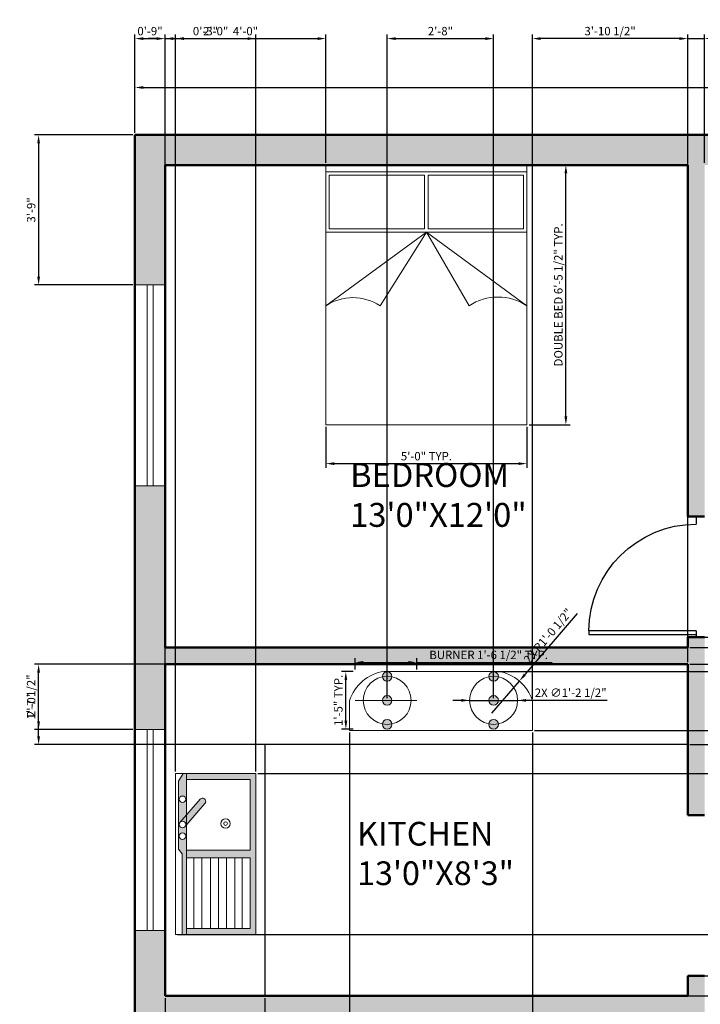
# Model space of a CAD drawing. Units: inches. Extents: x 457 to 882, y 0 to 1111.
# Tile 3 of 4: x 457 to 660, y 817 to 1111. Entities that reach past the tile are written whole.
import ezdxf

# ---------------------------------------------------------------- set-up
doc = ezdxf.new("R2010")
doc.units = ezdxf.units.IN
for name, color, linetype, lineweight in [('A-ANNO-DIMS', 2, 'Continuous', 18), ('A-AREA-IDEN', 7, 'Continuous', 25), ('A-DOOR', 3, 'Continuous', 25), ('A-EQPM', 9, 'Continuous', 18), ('A-FLOR-CASE', 8, 'Continuous', 25), ('A-FLOR-FIXT', 8, 'Continuous', 18), ('A-FLOR-FIXT-PATT', 8, 'Continuous', 13), ('A-FURN', 8, 'Continuous', 18), ('A-GLAZ', 5, 'Continuous', 18), ('A-WALL', 7, 'Continuous', 50), ('A-WALL-PATT', 252, 'Continuous', 13)]:
    doc.layers.add(name, color=color, linetype=linetype, lineweight=lineweight)
doc.styles.get("Standard").update_dxf_attribs({"font": 'arial.ttf'})
doc.dimstyles.new('ISO-25', dxfattribs={"dimtxt": 2.5, "dimasz": 2.5, "dimexe": 1.25, "dimexo": 0.625, "dimtad": 1, "dimdec": 0, "dimlunit": 3, "dimtxsty": 'Standard', "dimcen": 2.5, "dimadec": 0, "dimazin": 0, "dimtfac": 1, "dimtdec": 0, "dimtmove": 0, "dimatfit": 3, "dimfxl": 1, "dimarcsym": 0})

# ---------------------------------------------------------------- blocks, each defined once
blk = doc.blocks.new('*D2')
at = {"layer": 'A-ANNO-DIMS', "color": 0, "lineweight": -2, "transparency": 16777216}
for p, q in [((491.26, 1077.13), (491.26, 1091.91)), ((493.76, 1090.66), (848.76, 1090.66)), ((851.26, 1077.13), (851.26, 1091.91))]:
    blk.add_line(p, q, dxfattribs=at)
at = {"layer": 'A-ANNO-DIMS', "color": 0, "transparency": 16777216}
for points in [[(493.76, 1091.08), (493.76, 1090.24), (491.26, 1090.66)], [(848.76, 1091.08), (848.76, 1090.24), (851.26, 1090.66)]]:
    blk.add_solid(points, dxfattribs=at)
at = {"layer": 'Defpoints', "color": 0, "transparency": 16777216}
for p in [(851.26, 1090.66), (491.26, 1076.51), (851.26, 1076.51)]:
    blk.add_point(p, dxfattribs=at)
at = {"layer": 'A-ANNO-DIMS', "color": 0, "transparency": 16777216, "insert": (671.26, 1092.56), "char_height": 2.5, "attachment_point": 5}
blk.add_mtext("30'", dxfattribs=at)
blk = doc.blocks.new('BED-DOUBLE-60')
for p, q in [((0, 77.49), (0, 0)), ((60, 77.49), (0, 77.49)), ((60, 0), (60, 77.49)), ((60, 75.49), (0, 75.49)), ((29.44, 74.49), (0.94, 74.49)), ((0.94, 74.49), (0.94, 58.49)), ((29.44, 74.49), (29.44, 58.49)), ((59, 74.49), (30.53, 74.49)), ((30.53, 74.49), (30.53, 58.49)), ((59, 74.49), (59, 58.49)), ((60, 57.49), (0, 57.49)), ((30, 57.49), (0, 35.49)), ((29.44, 58.49), (0.94, 58.49)), ((30, 57.49), (16.16, 35.49)), ((60, 35.49), (30, 57.49)), ((30, 57.49), (42.73, 35.49)), ((59, 58.49), (30.53, 58.49)), ((0, 0), (60, 0))]:
    blk.add_line(p, q)
for centre, radius, start, end in [((8.08, 23.34), 14.59, 56.3669, 123.6331), ((51.36, 22.4), 15.69, 56.5972, 123.4028)]:
    blk.add_arc(centre, radius, start, end)
blk = doc.blocks.new('WIN-60-GLAZING')
for p, q in [((0, 0), (0, 60)), ((1.86, 0), (1.86, 60))]:
    blk.add_line(p, q)
blk = doc.blocks.new('DOOR-32-SWING')
for p, q in [((0, 36), (0, 33.7)), ((0, 1.85), (32, 1.85)), ((0, 1.85), (0, 0))]:
    blk.add_line(p, q)
blk.add_arc((0, 1.7), 32, 0.2643, 90)
blk = doc.blocks.new('COOKTOP-BURNER')
for q in [(0, 8.58), (18.39, 8.58)]:
    blk.add_line((9.57, 8.58), q)
for centre, radius in [((9.57, 8.58), 7.15), ((9.57, 15.73), 1.43), ((9.57, 8.58), 1.43), ((9.57, 1.43), 1.43)]:
    blk.add_circle(centre, radius)
blk = doc.blocks.new('*D16')
at = {"layer": 'A-ANNO-DIMS', "color": 0, "lineweight": -2, "transparency": 16777216}
for p, q in [((608.88, 1067.51), (621.13, 1067.51)), ((619.88, 992.51), (619.88, 1065.01)), ((608.88, 990.01), (621.13, 990.01))]:
    blk.add_line(p, q, dxfattribs=at)
at = {"layer": 'A-ANNO-DIMS', "color": 0, "transparency": 16777216}
for points in [[(619.46, 1065.01), (620.3, 1065.01), (619.88, 1067.51)], [(619.46, 992.51), (620.3, 992.51), (619.88, 990.01)]]:
    blk.add_solid(points, dxfattribs=at)
at = {"layer": 'Defpoints', "color": 0, "transparency": 16777216}
for p in [(608.26, 1067.51), (619.88, 1067.51), (608.26, 990.01)]:
    blk.add_point(p, dxfattribs=at)
at = {"layer": 'A-ANNO-DIMS', "color": 0, "transparency": 16777216, "insert": (617.96, 1028.76), "char_height": 2.5, "attachment_point": 5, "rotation": 90}
blk.add_mtext('DOUBLE BED 6\'-5 1/2" TYP.', dxfattribs=at)
blk = doc.blocks.new('*D17')
at = {"layer": 'A-ANNO-DIMS', "color": 0, "lineweight": -2, "transparency": 16777216}
for p, q in [((548.26, 989.39), (548.26, 977.14)), ((608.26, 989.39), (608.26, 977.14)), ((550.76, 978.39), (605.76, 978.39))]:
    blk.add_line(p, q, dxfattribs=at)
at = {"layer": 'A-ANNO-DIMS', "color": 0, "transparency": 16777216}
for points in [[(550.76, 978.8), (550.76, 977.97), (548.26, 978.39)], [(605.76, 978.8), (605.76, 977.97), (608.26, 978.39)]]:
    blk.add_solid(points, dxfattribs=at)
at = {"layer": 'Defpoints', "color": 0, "transparency": 16777216}
for p in [(548.26, 990.01), (608.26, 990.01), (608.26, 978.39)]:
    blk.add_point(p, dxfattribs=at)
at = {"layer": 'A-ANNO-DIMS', "color": 0, "transparency": 16777216, "insert": (578.26, 980.29), "char_height": 2.5, "attachment_point": 5}
blk.add_mtext('5\'-0" TYP.', dxfattribs=at)
blk = doc.blocks.new('*D22')
at = {"layer": 'A-ANNO-DIMS', "color": 0, "lineweight": -2, "transparency": 16777216}
for p, q in [((556.97, 916.92), (556.97, 920.31)), ((575.37, 916.92), (575.37, 920.31)), ((559.47, 919.06), (572.87, 919.06)), ((575.37, 919.06), (615.79, 919.06))]:
    blk.add_line(p, q, dxfattribs=at)
at = {"layer": 'A-ANNO-DIMS', "color": 0, "transparency": 16777216}
for points in [[(559.47, 919.48), (559.47, 918.64), (556.97, 919.06)], [(572.87, 919.48), (572.87, 918.64), (575.37, 919.06)]]:
    blk.add_solid(points, dxfattribs=at)
at = {"layer": 'Defpoints', "color": 0, "transparency": 16777216}
for p in [(575.37, 919.06), (556.97, 916.3), (575.37, 916.3)]:
    blk.add_point(p, dxfattribs=at)
at = {"layer": 'A-ANNO-DIMS', "color": 0, "transparency": 16777216, "insert": (596.83, 920.98), "char_height": 2.5, "attachment_point": 5}
blk.add_mtext('BURNER 1\'-6 1/2" TYP.', dxfattribs=at)
blk = doc.blocks.new('*D23')
at = {"layer": 'A-ANNO-DIMS', "color": 0, "lineweight": -2, "transparency": 16777216}
for p, q in [((556.35, 916.3), (552.96, 916.3)), ((554.21, 901.64), (554.21, 913.8)), ((556.35, 899.14), (552.96, 899.14))]:
    blk.add_line(p, q, dxfattribs=at)
at = {"layer": 'A-ANNO-DIMS', "color": 0, "transparency": 16777216}
for points in [[(553.8, 913.8), (554.63, 913.8), (554.21, 916.3)], [(553.8, 901.64), (554.63, 901.64), (554.21, 899.14)]]:
    blk.add_solid(points, dxfattribs=at)
at = {"layer": 'Defpoints', "color": 0, "transparency": 16777216}
for p in [(554.21, 916.3), (556.97, 916.3), (556.97, 899.14)]:
    blk.add_point(p, dxfattribs=at)
at = {"layer": 'A-ANNO-DIMS', "color": 0, "transparency": 16777216, "insert": (552.31, 907.72), "char_height": 2.5, "attachment_point": 5, "rotation": 90}
blk.add_mtext('1\'-5" TYP.', dxfattribs=at)
blk = doc.blocks.new('*D27')
at = {"layer": 'A-ANNO-DIMS', "color": 0, "lineweight": -2, "transparency": 16777216}
for p, q in [((685.01, 929.13), (685.01, 931.63)), ((656.88, 926.63), (686.26, 926.63)), ((685.01, 926.63), (685.01, 923.51)), ((656.88, 923.51), (686.26, 923.51)), ((685.01, 921.01), (685.01, 910.61))]:
    blk.add_line(p, q, dxfattribs=at)
at = {"layer": 'A-ANNO-DIMS', "color": 0, "transparency": 16777216}
for points in [[(684.59, 929.13), (685.42, 929.13), (685.01, 926.63)], [(684.59, 921.01), (685.42, 921.01), (685.01, 923.51)]]:
    blk.add_solid(points, dxfattribs=at)
at = {"layer": 'Defpoints', "color": 0, "transparency": 16777216}
for p in [(656.26, 926.63), (656.26, 923.51), (685.01, 923.51)]:
    blk.add_point(p, dxfattribs=at)
at = {"layer": 'A-ANNO-DIMS', "color": 0, "transparency": 16777216, "insert": (683.11, 914.56), "char_height": 2.5, "attachment_point": 5, "rotation": 90}
blk.add_mtext('0\'-3"', dxfattribs=at)
blk = doc.blocks.new('*D28')
at = {"layer": 'A-ANNO-DIMS', "color": 0, "lineweight": -2, "transparency": 16777216}
for p, q in [((491.26, 1077.13), (491.26, 1106.51)), ((493.76, 1105.26), (497.76, 1105.26)), ((500.26, 1068.13), (500.26, 1106.51))]:
    blk.add_line(p, q, dxfattribs=at)
at = {"layer": 'A-ANNO-DIMS', "color": 0, "transparency": 16777216}
for points in [[(493.76, 1105.67), (493.76, 1104.84), (491.26, 1105.26)], [(497.76, 1105.67), (497.76, 1104.84), (500.26, 1105.26)]]:
    blk.add_solid(points, dxfattribs=at)
at = {"layer": 'Defpoints', "color": 0, "transparency": 16777216}
for p in [(500.26, 1105.26), (491.26, 1076.51), (500.26, 1067.51)]:
    blk.add_point(p, dxfattribs=at)
at = {"layer": 'A-ANNO-DIMS', "color": 0, "transparency": 16777216, "insert": (495.76, 1107.16), "char_height": 2.5, "attachment_point": 5}
blk.add_mtext('0\'-9"', dxfattribs=at)
blk = doc.blocks.new('*D29')
at = {"layer": 'A-ANNO-DIMS', "color": 0, "lineweight": -2, "transparency": 16777216}
for p, q in [((653.76, 1105.26), (651.26, 1105.26)), ((656.26, 1068.13), (656.26, 1106.51)), ((656.26, 1105.26), (661.26, 1105.26)), ((661.26, 1068.13), (661.26, 1106.51)), ((663.76, 1105.26), (674.15, 1105.26))]:
    blk.add_line(p, q, dxfattribs=at)
at = {"layer": 'A-ANNO-DIMS', "color": 0, "transparency": 16777216}
for points in [[(653.76, 1105.67), (653.76, 1104.84), (656.26, 1105.26)], [(663.76, 1105.67), (663.76, 1104.84), (661.26, 1105.26)]]:
    blk.add_solid(points, dxfattribs=at)
at = {"layer": 'Defpoints', "color": 0, "transparency": 16777216}
for p in [(661.26, 1105.26), (656.26, 1067.51), (661.26, 1067.51)]:
    blk.add_point(p, dxfattribs=at)
at = {"layer": 'A-ANNO-DIMS', "color": 0, "transparency": 16777216, "insert": (670.21, 1107.16), "char_height": 2.5, "attachment_point": 5}
blk.add_mtext('0\'-5"', dxfattribs=at)
blk = doc.blocks.new('*D30')
at = {"layer": 'A-ANNO-DIMS', "color": 0, "lineweight": -2, "transparency": 16777216}
for p, q in [((490.63, 1076.51), (461.26, 1076.51)), ((462.51, 1074.01), (462.51, 1034.23)), ((490.63, 1031.73), (461.26, 1031.73))]:
    blk.add_line(p, q, dxfattribs=at)
at = {"layer": 'A-ANNO-DIMS', "color": 0, "transparency": 16777216}
for points in [[(462.09, 1074.01), (462.92, 1074.01), (462.51, 1076.51)], [(462.09, 1034.23), (462.92, 1034.23), (462.51, 1031.73)]]:
    blk.add_solid(points, dxfattribs=at)
at = {"layer": 'Defpoints', "color": 0, "transparency": 16777216}
for p in [(491.26, 1076.51), (462.51, 1031.73), (491.26, 1031.73)]:
    blk.add_point(p, dxfattribs=at)
at = {"layer": 'A-ANNO-DIMS', "color": 0, "transparency": 16777216, "insert": (460.61, 1054.12), "char_height": 2.5, "attachment_point": 5, "rotation": 90}
blk.add_mtext('3\'-9"', dxfattribs=at)
blk = doc.blocks.new('*D31')
at = {"layer": 'A-ANNO-DIMS', "color": 0, "lineweight": -2, "transparency": 16777216}
for p, q in [((499.63, 918.51), (461.26, 918.51)), ((462.51, 901.51), (462.51, 916.01)), ((490.63, 899.01), (461.26, 899.01))]:
    blk.add_line(p, q, dxfattribs=at)
at = {"layer": 'A-ANNO-DIMS', "color": 0, "transparency": 16777216}
for points in [[(462.09, 916.01), (462.92, 916.01), (462.51, 918.51)], [(462.09, 901.51), (462.92, 901.51), (462.51, 899.01)]]:
    blk.add_solid(points, dxfattribs=at)
at = {"layer": 'Defpoints', "color": 0, "transparency": 16777216}
for p in [(462.51, 918.51), (500.26, 918.51), (491.26, 899.01)]:
    blk.add_point(p, dxfattribs=at)
at = {"layer": 'A-ANNO-DIMS', "color": 0, "transparency": 16777216, "insert": (460.59, 908.76), "char_height": 2.5, "attachment_point": 5, "rotation": 90}
blk.add_mtext('1\'-7 1/2"', dxfattribs=at)
blk = doc.blocks.new('*D45')
at = {"layer": 'A-ANNO-DIMS', "color": 0, "lineweight": -2, "transparency": 16777216}
for p, q in [((500.26, 818.88), (500.26, 506.51)), ((530, 818.88), (530, 506.51)), ((502.76, 507.76), (527.5, 507.76))]:
    blk.add_line(p, q, dxfattribs=at)
at = {"layer": 'A-ANNO-DIMS', "color": 0, "transparency": 16777216}
for points in [[(502.76, 508.17), (502.76, 507.34), (500.26, 507.76)], [(527.5, 508.17), (527.5, 507.34), (530, 507.76)]]:
    blk.add_solid(points, dxfattribs=at)
at = {"layer": 'Defpoints', "color": 0, "transparency": 16777216}
for p in [(500.26, 819.51), (530, 819.51), (530, 507.76)]:
    blk.add_point(p, dxfattribs=at)
at = {"layer": 'A-ANNO-DIMS', "color": 0, "transparency": 16777216, "insert": (515.13, 509.67), "char_height": 2.5, "attachment_point": 5}
blk.add_mtext('2\'-5 1/2"', dxfattribs=at)
blk = doc.blocks.new('*D46')
at = {"layer": 'A-ANNO-DIMS', "color": 0, "lineweight": -2, "transparency": 16777216}
for p, q in [((655.63, 918.51), (461.26, 918.51)), ((462.51, 897.01), (462.51, 916.01)), ((655.63, 894.51), (461.26, 894.51))]:
    blk.add_line(p, q, dxfattribs=at)
at = {"layer": 'A-ANNO-DIMS', "color": 0, "transparency": 16777216}
for points in [[(462.09, 916.01), (462.92, 916.01), (462.51, 918.51)], [(462.09, 897.01), (462.92, 897.01), (462.51, 894.51)]]:
    blk.add_solid(points, dxfattribs=at)
at = {"layer": 'Defpoints', "color": 0, "transparency": 16777216}
for p in [(462.51, 918.51), (656.26, 918.51), (656.26, 894.51)]:
    blk.add_point(p, dxfattribs=at)
at = {"layer": 'A-ANNO-DIMS', "color": 0, "transparency": 16777216, "insert": (460.61, 906.51), "char_height": 2.5, "attachment_point": 5, "rotation": 90}
blk.add_mtext('2\'-0"', dxfattribs=at)
blk = doc.blocks.new('*D48')
at = {"layer": 'A-ANNO-DIMS', "color": 0, "lineweight": -2, "transparency": 16777216}
for p, q in [((880.01, 828.01), (880.01, 838.4)), ((656.88, 825.51), (881.26, 825.51)), ((880.01, 819.51), (880.01, 825.51)), ((656.88, 819.51), (881.26, 819.51)), ((880.01, 817.01), (880.01, 814.51))]:
    blk.add_line(p, q, dxfattribs=at)
at = {"layer": 'A-ANNO-DIMS', "color": 0, "transparency": 16777216}
for points in [[(879.59, 828.01), (880.42, 828.01), (880.01, 825.51)], [(879.59, 817.01), (880.42, 817.01), (880.01, 819.51)]]:
    blk.add_solid(points, dxfattribs=at)
at = {"layer": 'Defpoints', "color": 0, "transparency": 16777216}
for p in [(656.26, 825.51), (880.01, 825.51), (656.26, 819.51)]:
    blk.add_point(p, dxfattribs=at)
at = {"layer": 'A-ANNO-DIMS', "color": 0, "transparency": 16777216, "insert": (878.11, 834.45), "char_height": 2.5, "attachment_point": 5, "rotation": 90}
blk.add_mtext('0\'-6"', dxfattribs=at)
blk = doc.blocks.new('*D49')
at = {"layer": 'A-ANNO-DIMS', "color": 0, "lineweight": -2, "transparency": 16777216}
for p, q in [((503.36, 886.5), (503.36, 1106.51)), ((505.86, 1105.26), (524.86, 1105.26)), ((527.36, 886.5), (527.36, 1106.51))]:
    blk.add_line(p, q, dxfattribs=at)
at = {"layer": 'A-ANNO-DIMS', "color": 0, "transparency": 16777216}
for points in [[(505.86, 1105.67), (505.86, 1104.84), (503.36, 1105.26)], [(524.86, 1105.67), (524.86, 1104.84), (527.36, 1105.26)]]:
    blk.add_solid(points, dxfattribs=at)
at = {"layer": 'Defpoints', "color": 0, "transparency": 16777216}
for p in [(527.36, 1105.26), (503.36, 885.87), (527.36, 885.87)]:
    blk.add_point(p, dxfattribs=at)
at = {"layer": 'A-ANNO-DIMS', "color": 0, "transparency": 16777216, "insert": (515.36, 1107.16), "char_height": 2.5, "attachment_point": 5}
blk.add_mtext('2\'-0"', dxfattribs=at)
blk = doc.blocks.new('*D50')
at = {"layer": 'A-ANNO-DIMS', "color": 0, "lineweight": -2, "transparency": 16777216}
for p, q in [((527.99, 885.87), (881.26, 885.87)), ((880.01, 840.37), (880.01, 883.37)), ((527.99, 837.87), (881.26, 837.87))]:
    blk.add_line(p, q, dxfattribs=at)
at = {"layer": 'A-ANNO-DIMS', "color": 0, "transparency": 16777216}
for points in [[(879.59, 883.37), (880.42, 883.37), (880.01, 885.87)], [(879.59, 840.37), (880.42, 840.37), (880.01, 837.87)]]:
    blk.add_solid(points, dxfattribs=at)
at = {"layer": 'Defpoints', "color": 0, "transparency": 16777216}
for p in [(527.36, 885.87), (880.01, 885.87), (527.36, 837.87)]:
    blk.add_point(p, dxfattribs=at)
at = {"layer": 'A-ANNO-DIMS', "color": 0, "transparency": 16777216, "insert": (878.11, 861.87), "char_height": 2.5, "attachment_point": 5, "rotation": 90}
blk.add_mtext('4\'-0"', dxfattribs=at)
blk = doc.blocks.new('*D51')
at = {"layer": 'A-ANNO-DIMS', "color": 0, "lineweight": -2, "transparency": 16777216}
for p, q in [((503.99, 837.87), (881.26, 837.87)), ((880.01, 822.01), (880.01, 835.37)), ((500.88, 819.51), (881.26, 819.51))]:
    blk.add_line(p, q, dxfattribs=at)
at = {"layer": 'A-ANNO-DIMS', "color": 0, "transparency": 16777216}
for points in [[(879.59, 835.37), (880.42, 835.37), (880.01, 837.87)], [(879.59, 822.01), (880.42, 822.01), (880.01, 819.51)]]:
    blk.add_solid(points, dxfattribs=at)
at = {"layer": 'Defpoints', "color": 0, "transparency": 16777216}
for p in [(503.36, 837.87), (880.01, 837.87), (500.26, 819.51)]:
    blk.add_point(p, dxfattribs=at)
at = {"layer": 'A-ANNO-DIMS', "color": 0, "transparency": 16777216, "insert": (878.09, 828.69), "char_height": 2.5, "attachment_point": 5, "rotation": 90}
blk.add_mtext('1\'-6 1/2"', dxfattribs=at)
blk = doc.blocks.new('*D52')
at = {"layer": 'A-ANNO-DIMS', "color": 0, "lineweight": -2, "transparency": 16777216}
for p, q in [((497.76, 1105.26), (495.26, 1105.26)), ((500.26, 899.63), (500.26, 1106.51)), ((500.26, 1105.26), (503.36, 1105.26)), ((503.36, 886.5), (503.36, 1106.51)), ((505.86, 1105.26), (516.26, 1105.26))]:
    blk.add_line(p, q, dxfattribs=at)
at = {"layer": 'A-ANNO-DIMS', "color": 0, "transparency": 16777216}
for points in [[(497.76, 1105.67), (497.76, 1104.84), (500.26, 1105.26)], [(505.86, 1105.67), (505.86, 1104.84), (503.36, 1105.26)]]:
    blk.add_solid(points, dxfattribs=at)
at = {"layer": 'Defpoints', "color": 0, "transparency": 16777216}
for p in [(503.36, 1105.26), (500.26, 899.01), (503.36, 885.87)]:
    blk.add_point(p, dxfattribs=at)
at = {"layer": 'A-ANNO-DIMS', "color": 0, "transparency": 16777216, "insert": (512.31, 1107.16), "char_height": 2.5, "attachment_point": 5}
blk.add_mtext('0\'-3"', dxfattribs=at)
blk = doc.blocks.new('*D53')
at = {"layer": 'A-ANNO-DIMS', "color": 0, "lineweight": -2, "transparency": 16777216}
for p, q in [((566.55, 908.35), (566.55, 1106.51)), ((569.05, 1105.26), (595.81, 1105.26)), ((598.31, 908.35), (598.31, 1106.51))]:
    blk.add_line(p, q, dxfattribs=at)
at = {"layer": 'A-ANNO-DIMS', "color": 0, "transparency": 16777216}
for points in [[(569.05, 1105.67), (569.05, 1104.84), (566.55, 1105.26)], [(595.81, 1105.67), (595.81, 1104.84), (598.31, 1105.26)]]:
    blk.add_solid(points, dxfattribs=at)
at = {"layer": 'Defpoints', "color": 0, "transparency": 16777216}
for p in [(598.31, 1105.26), (566.55, 907.72), (598.31, 907.72)]:
    blk.add_point(p, dxfattribs=at)
at = {"layer": 'A-ANNO-DIMS', "color": 0, "transparency": 16777216, "insert": (582.43, 1107.16), "char_height": 2.5, "attachment_point": 5}
blk.add_mtext('2\'-8"', dxfattribs=at)
blk = doc.blocks.new('*D54')
at = {"layer": 'A-ANNO-DIMS', "color": 0, "lineweight": -2, "transparency": 16777216}
for p, q in [((609.9, 908.2), (609.9, 1106.51)), ((653.76, 1105.26), (612.4, 1105.26)), ((656.26, 919.13), (656.26, 1106.51))]:
    blk.add_line(p, q, dxfattribs=at)
at = {"layer": 'A-ANNO-DIMS', "color": 0, "transparency": 16777216}
for points in [[(612.4, 1105.67), (612.4, 1104.84), (609.9, 1105.26)], [(653.76, 1105.67), (653.76, 1104.84), (656.26, 1105.26)]]:
    blk.add_solid(points, dxfattribs=at)
at = {"layer": 'Defpoints', "color": 0, "transparency": 16777216}
for p in [(609.9, 1105.26), (656.26, 918.51), (609.9, 907.58)]:
    blk.add_point(p, dxfattribs=at)
at = {"layer": 'A-ANNO-DIMS', "color": 0, "transparency": 16777216, "insert": (633.08, 1107.17), "char_height": 2.5, "attachment_point": 5}
blk.add_mtext('3\'-10 1/2"', dxfattribs=at)
blk = doc.blocks.new('*D55')
at = {"layer": 'A-ANNO-DIMS', "color": 0, "lineweight": -2, "transparency": 16777216}
for p, q in [((880.01, 921.01), (880.01, 931.4)), ((656.88, 918.51), (881.26, 918.51)), ((880.01, 916.3), (880.01, 918.51)), ((598.94, 916.3), (881.26, 916.3)), ((880.01, 913.8), (880.01, 911.3))]:
    blk.add_line(p, q, dxfattribs=at)
at = {"layer": 'A-ANNO-DIMS', "color": 0, "transparency": 16777216}
for points in [[(879.59, 921.01), (880.42, 921.01), (880.01, 918.51)], [(879.59, 913.8), (880.42, 913.8), (880.01, 916.3)]]:
    blk.add_solid(points, dxfattribs=at)
at = {"layer": 'Defpoints', "color": 0, "transparency": 16777216}
for p in [(656.26, 918.51), (880.01, 918.51), (598.31, 916.3)]:
    blk.add_point(p, dxfattribs=at)
at = {"layer": 'A-ANNO-DIMS', "color": 0, "transparency": 16777216, "insert": (878.11, 927.45), "char_height": 2.5, "attachment_point": 5, "rotation": 90}
blk.add_mtext('0\'-2"', dxfattribs=at)
blk = doc.blocks.new('*D56')
at = {"layer": 'A-ANNO-DIMS', "color": 0, "lineweight": -2, "transparency": 16777216}
for p, q in [((555.33, 898.14), (555.33, 506.51)), ((609.9, 898.14), (609.9, 506.51)), ((557.83, 507.76), (607.4, 507.76))]:
    blk.add_line(p, q, dxfattribs=at)
at = {"layer": 'A-ANNO-DIMS', "color": 0, "transparency": 16777216}
for points in [[(557.83, 508.17), (557.83, 507.34), (555.33, 507.76)], [(607.4, 508.17), (607.4, 507.34), (609.9, 507.76)]]:
    blk.add_solid(points, dxfattribs=at)
at = {"layer": 'Defpoints', "color": 0, "transparency": 16777216}
for p in [(555.33, 898.77), (609.9, 898.77), (609.9, 507.76)]:
    blk.add_point(p, dxfattribs=at)
at = {"layer": 'A-ANNO-DIMS', "color": 0, "transparency": 16777216, "insert": (582.61, 509.67), "char_height": 2.5, "attachment_point": 5}
blk.add_mtext('4\'-6 1/2"', dxfattribs=at)
blk = doc.blocks.new('*D57')
at = {"layer": 'A-ANNO-DIMS', "color": 0, "lineweight": -2, "transparency": 16777216}
for p, q in [((880.01, 901.27), (880.01, 903.77)), ((610.53, 898.77), (881.26, 898.77)), ((880.01, 898.77), (880.01, 894.51)), ((656.88, 894.51), (881.26, 894.51)), ((880.01, 892.01), (880.01, 875.78))]:
    blk.add_line(p, q, dxfattribs=at)
at = {"layer": 'A-ANNO-DIMS', "color": 0, "transparency": 16777216}
for points in [[(879.59, 901.27), (880.42, 901.27), (880.01, 898.77)], [(879.59, 892.01), (880.42, 892.01), (880.01, 894.51)]]:
    blk.add_solid(points, dxfattribs=at)
at = {"layer": 'Defpoints', "color": 0, "transparency": 16777216}
for p in [(609.9, 898.77), (656.26, 894.51), (880.01, 894.51)]:
    blk.add_point(p, dxfattribs=at)
at = {"layer": 'A-ANNO-DIMS', "color": 0, "transparency": 16777216, "insert": (878.09, 882.64), "char_height": 2.5, "attachment_point": 5, "rotation": 90}
blk.add_mtext('0\'-4 1/2"', dxfattribs=at)
blk = doc.blocks.new('*D58')
at = {"layer": 'A-ANNO-DIMS', "color": 0, "lineweight": -2, "transparency": 16777216}
for p, q in [((500.26, 1068.13), (500.26, 1106.51)), ((502.76, 1105.26), (545.76, 1105.26)), ((548.26, 1068.13), (548.26, 1106.51))]:
    blk.add_line(p, q, dxfattribs=at)
at = {"layer": 'A-ANNO-DIMS', "color": 0, "transparency": 16777216}
for points in [[(502.76, 1105.67), (502.76, 1104.84), (500.26, 1105.26)], [(545.76, 1105.67), (545.76, 1104.84), (548.26, 1105.26)]]:
    blk.add_solid(points, dxfattribs=at)
at = {"layer": 'Defpoints', "color": 0, "transparency": 16777216}
for p in [(548.26, 1105.26), (500.26, 1067.51), (548.26, 1067.51)]:
    blk.add_point(p, dxfattribs=at)
at = {"layer": 'A-ANNO-DIMS', "color": 0, "transparency": 16777216, "insert": (524.26, 1107.16), "char_height": 2.5, "attachment_point": 5}
blk.add_mtext('4\'-0"', dxfattribs=at)
blk = doc.blocks.new('*D63')
at = {"layer": 'A-ANNO-DIMS', "color": 0, "lineweight": -2, "transparency": 16777216}
for p, q in [((588.66, 907.72), (586.16, 907.72)), ((591.16, 907.72), (605.46, 907.72)), ((632.18, 907.72), (607.96, 907.72))]:
    blk.add_line(p, q, dxfattribs=at)
at = {"layer": 'A-ANNO-DIMS', "color": 0, "transparency": 16777216}
for points in [[(588.66, 908.14), (588.66, 907.31), (591.16, 907.72)], [(607.96, 908.14), (607.96, 907.31), (605.46, 907.72)]]:
    blk.add_solid(points, dxfattribs=at)
at = {"layer": 'Defpoints', "color": 0, "transparency": 16777216}
for p in [(591.16, 907.72), (605.46, 907.72)]:
    blk.add_point(p, dxfattribs=at)
at = {"layer": 'A-ANNO-DIMS', "color": 0, "transparency": 16777216, "insert": (621.32, 909.69), "char_height": 2.5, "attachment_point": 5, "rotation": 359.9999}
blk.add_mtext('2X ∅1\'-2 1/2"', dxfattribs=at)
blk = doc.blocks.new('*D64')
at = {"layer": 'A-ANNO-DIMS', "color": 0, "lineweight": -2, "transparency": 16777216}
for p, q in [((623.21, 933.69), (607.63, 915.4)), ((597.82, 903.87), (606.01, 913.49))]:
    blk.add_line(p, q, dxfattribs=at)
at = {"layer": 'A-ANNO-DIMS', "color": 0, "transparency": 16777216}
blk.add_solid([(607.31, 915.67), (607.95, 915.13), (606.01, 913.49)], dxfattribs=at)
at = {"layer": 'Defpoints', "color": 0, "transparency": 16777216}
for p in [(606.01, 913.49), (597.82, 903.87)]:
    blk.add_point(p, dxfattribs=at)
at = {"layer": 'A-ANNO-DIMS', "color": 0, "transparency": 16777216, "insert": (614.77, 926.74), "char_height": 2.5, "attachment_point": 5, "rotation": 49.5942}
blk.add_mtext('2X R1\'-0 1/2"', dxfattribs=at)

msp = doc.modelspace()

# ---------------------------------------------------------------- hatches: boundary and pattern name
at = {"layer": 'A-FLOR-FIXT-PATT'}
h = msp.add_hatch(color=256, dxfattribs=at)
h.dxf.hatch_style = 1
h.paths.add_polyline_path([(527.36, 885.87), (506.68, 885.87), (506.68, 884.15), (525.64, 884.15), (525.64, 863), (506.68, 863), (506.68, 860.72), (525.64, 860.72), (525.64, 839.59), (506.68, 839.59), (506.68, 837.87), (527.36, 837.87)])
h.paths.add_polyline_path([(506.68, 870.61), (506.22, 870.07, -0.7167), (504.48, 870.66, -0.191592), (504.75, 871.32), (506.68, 873.57), (506.68, 885.87), (505.66, 885.87), (504.26, 883.63), (504.26, 863.31), (505.39, 861.92), (505.39, 837.87), (506.68, 837.87), (506.68, 839.59), (506.68, 863)])
h.paths.add_polyline_path([(504.48, 867.19, -1), (506.42, 867.19, -1)], flags=16)
h.paths.add_polyline_path([(504.48, 878.2, -1), (506.42, 878.2, -1)], flags=16)
h.paths.add_polyline_path([(567.97, 914.73, 0.10044), (565.12, 914.73, 0.904592)])
h.paths.add_polyline_path([(565.12, 914.87, 0.025031), (565.12, 914.73, -0.10044), (567.97, 914.73, 0.025031), (567.98, 914.87, 1)])
h.paths.add_polyline_path([(565.12, 907.72), (566.55, 907.72), (567.98, 907.72, 1)])
h.paths.add_polyline_path([(567.98, 907.72), (566.55, 907.72), (565.12, 907.72, 1)])
h.paths.add_polyline_path([(565.12, 900.72, 0.10044), (567.97, 900.72, 0.904592)])
h.paths.add_polyline_path([(567.98, 900.57, 0.025031), (567.97, 900.72, -0.10044), (565.12, 900.72, 0.025031), (565.12, 900.57, 1)])
h.paths.add_polyline_path([(596.88, 907.72), (598.31, 907.72), (599.74, 907.72, 1)])
h.paths.add_polyline_path([(599.74, 907.72), (598.31, 907.72), (596.88, 907.72, 1)])
h.paths.add_polyline_path([(596.88, 914.87, 0.025031), (596.89, 914.73, -0.10044), (599.73, 914.73, 0.025031), (599.74, 914.87, 1)])
h.paths.add_polyline_path([(599.73, 914.73, 0.10044), (596.89, 914.73, 0.904592)])
h.paths.add_polyline_path([(596.89, 900.72, 0.10044), (599.73, 900.72, 0.904592)])
h.paths.add_polyline_path([(599.74, 900.57, 0.025031), (599.73, 900.72, -0.10044), (596.89, 900.72, 0.025031), (596.88, 900.57, 1)])
h = msp.add_hatch(color=256, dxfattribs=at)
h.dxf.hatch_style = 1
h.paths.add_polyline_path([(512.13, 876.94, 1), (510.68, 878.21), (506.68, 873.57), (506.68, 870.61)])
h.paths.add_polyline_path([(506.68, 873.57), (504.75, 871.32, -0.678427), (506.42, 870.66, -0.165026), (506.22, 870.07), (506.68, 870.61)])
at = {"layer": 'A-WALL-PATT'}
h = msp.add_hatch(color=256, dxfattribs=at)
h.dxf.hatch_style = 1
h.paths.add_polyline_path([(677.26, 1076.51), (491.26, 1076.51), (491.26, 1031.73), (500.26, 1031.73), (500.26, 1067.51), (656.26, 1067.51), (656.26, 962.63), (661.26, 962.63), (661.26, 1067.51), (677.26, 1067.51)])
h.paths.add_polyline_path([(851.26, 1076.51), (701.26, 1076.51), (701.26, 1067.51), (717.26, 1067.51), (717.26, 971.51), (691.26, 971.51), (691.26, 966.51), (717.26, 966.51), (717.26, 962.63), (722.26, 962.63), (722.26, 1067.51), (842.26, 1067.51), (842.26, 1031.73), (851.26, 1031.73)])
h.paths.add_polyline_path([(851.26, 971.73), (842.26, 971.73), (842.26, 923.51), (722.26, 923.51), (722.26, 926.63), (717.26, 926.63), (717.26, 918.51), (842.26, 918.51), (842.26, 896.98), (851.26, 896.98)])
h.paths.add_polyline_path([(661.26, 926.63), (656.26, 926.63), (656.26, 923.51), (500.26, 923.51), (500.26, 971.73), (491.26, 971.73), (491.26, 899.01), (500.26, 899.01), (500.26, 918.51), (656.26, 918.51), (656.26, 873.51), (661.26, 873.51)])
h.paths.add_polyline_path([(500.26, 839.01), (491.26, 839.01), (491.26, 778.51), (500.26, 778.51), (500.26, 814.51), (656.26, 814.51), (656.26, 726.51), (661.26, 726.51), (661.26, 825.51), (656.26, 825.51), (656.26, 819.51), (500.26, 819.51)])
h.paths.add_polyline_path([(661.26, 633.51), (656.26, 633.51), (656.26, 545.51), (606.26, 545.51), (606.26, 536.51), (661.26, 536.51)], flags=0)
h.paths.add_polyline_path([(851.26, 560.51), (842.26, 560.51), (842.26, 545.51), (721.26, 545.51), (721.26, 536.51), (851.26, 536.51)])
h.paths.add_polyline_path([(851.26, 649.3), (842.26, 649.3), (842.26, 628.51), (700.26, 628.51), (700.26, 623.51), (842.26, 623.51), (842.26, 608.51), (851.26, 608.51)])
h.paths.add_polyline_path([(500.26, 677.51), (656.26, 677.51), (656.26, 671.51), (661.26, 671.51), (661.26, 688.51), (656.26, 688.51), (656.26, 682.51), (500.26, 682.51), (500.26, 718.51), (491.26, 718.51), (491.26, 536.51), (546.26, 536.51), (546.26, 545.51), (500.26, 545.51)])

# ---------------------------------------------------------------- linework, layer by layer
at = {"layer": 'A-DOOR'}
for p, q in [((626.76, 928.48), (626.76, 927.41)), ((626.76, 927.41), (658.76, 927.41))]:
    msp.add_line(p, q, dxfattribs=at)
at = {"layer": 'A-EQPM'}
for points in [[(599.55, 916.39), (565.68, 916.39)], [(555.33, 907.58), (555.33, 898.77), (609.9, 898.77), (609.9, 907.58)]]:
    msp.add_lwpolyline(points, dxfattribs=at)
for centre, start, end in [((567.41, 903.87), 97.8676, 162.9379), ((597.82, 903.87), 17.0621, 82.1324)]:
    msp.add_arc(centre, 12.64, start, end, dxfattribs=at)
at = {"layer": 'A-FLOR-CASE'}
for p, q in [((656.26, 894.51), (530, 894.51)), ((530, 894.51), (530, 819.51))]:
    msp.add_line(p, q, dxfattribs=at)
at = {"layer": 'A-FLOR-FIXT'}
for p, q in [((504.26, 883.63), (505.66, 885.87)), ((506.68, 885.87), (506.68, 839.59)), ((504.26, 863.31), (504.26, 883.63)), ((525.64, 884.15), (506.68, 884.15)), ((525.64, 863), (525.64, 884.15)), ((504.69, 871.25), (510.68, 878.21)), ((506.15, 869.99), (512.13, 876.94)), ((505.39, 861.92), (504.26, 863.31)), ((505.39, 837.87), (505.39, 861.92)), ((506.68, 863), (525.64, 863)), ((506.68, 863), (506.68, 837.87)), ((506.68, 860.72), (525.64, 860.72)), ((508.81, 860.72), (508.81, 839.59)), ((511.27, 860.72), (511.27, 839.59)), ((513.85, 860.72), (513.85, 839.59)), ((516.16, 860.72), (516.16, 839.59)), ((518.62, 860.72), (518.62, 839.59)), ((521.05, 860.72), (521.05, 839.59)), ((523.26, 860.72), (523.26, 839.59)), ((525.64, 839.59), (525.64, 860.72)), ((506.68, 839.59), (525.64, 839.59))]:
    msp.add_line(p, q, dxfattribs=at)
msp.add_lwpolyline([(527.36, 837.87), (527.36, 885.87), (503.36, 885.87), (503.36, 837.87)], close=True, dxfattribs=at)
for centre, radius in [((505.45, 878.2), 0.968), ((505.45, 870.66), 0.968), ((518.31, 870.95), 1.4), ((518.31, 870.95), 0.53), ((505.45, 867.19), 0.968)]:
    msp.add_circle(centre, radius, dxfattribs=at)
msp.add_arc((511.41, 877.57), 0.967, 318.6356, 139.8824, dxfattribs=at)
at = {"layer": 'A-GLAZ'}
for p, q in [((500.26, 1031.73), (491.26, 1031.73)), ((491.26, 971.73), (500.26, 971.73)), ((500.26, 899.01), (491.26, 899.01)), ((491.26, 839.01), (500.26, 839.01))]:
    msp.add_line(p, q, dxfattribs=at)
at = {"layer": 'A-WALL'}
for p, q in [((851.26, 1076.51), (491.26, 1076.51)), ((491.26, 1076.51), (491.26, 536.51)), ((500.26, 1067.51), (500.26, 923.51)), ((656.26, 1067.51), (500.26, 1067.51)), ((656.26, 1067.51), (656.26, 962.63)), ((661.26, 962.63), (656.26, 962.63)), ((661.26, 926.63), (656.26, 926.63)), ((656.26, 926.63), (656.26, 923.51)), ((656.26, 923.51), (500.26, 923.51)), ((500.26, 918.51), (500.26, 819.51)), ((656.26, 918.51), (500.26, 918.51)), ((656.26, 918.51), (656.26, 873.51)), ((656.26, 873.51), (661.26, 873.51)), ((656.26, 825.51), (661.26, 825.51)), ((656.26, 825.51), (656.26, 819.51)), ((500.26, 819.51), (656.26, 819.51))]:
    msp.add_line(p, q, dxfattribs=at)

# ---------------------------------------------------------------- block references
at = {"layer": 'A-DOOR', "extrusion": (0, 0, -1), "zscale": -1}
msp.add_blockref('DOOR-32-SWING', (-658.76, 926.63), dxfattribs=at)
at = {"layer": 'A-EQPM'}
for p in [(556.97, 899.14), (588.74, 899.14)]:
    msp.add_blockref('COOKTOP-BURNER', p, dxfattribs=at)
at = {"layer": 'A-FURN'}
msp.add_blockref('BED-DOUBLE-60', (548.26, 990.01), dxfattribs=at)
at = {"layer": 'A-GLAZ'}
for p in [(494.86, 971.73), (494.86, 839)]:
    msp.add_blockref('WIN-60-GLAZING', p, dxfattribs=at)

# ---------------------------------------------------------------- texts
at = {"layer": 'A-AREA-IDEN', "attachment_point": 1}
for s, width, gutter_width, insert, char_height in [('BEDROOM\\P13\'0"X12\'0"', 62.6238, 35.71, (555.51, 978.57), 7.1429), ('KITCHEN\\P13\'0"X8\'3"', 145.2671, 35.38, (557.56, 871.46), 7.075)]:
    msp.add_mtext_dynamic_manual_height_columns(s, width=width, gutter_width=gutter_width, heights=[0], dxfattribs=dict(at, insert=insert, char_height=char_height))

# ---------------------------------------------------------------- dimensions: what is measured, and where the dimension line sits
at = {"layer": 'A-ANNO-DIMS'}
for base, p1, p2, override, picture, middle in [((500.26, 1105.26), (491.26, 1076.51), (500.26, 1067.51), {"dimdec": 1, "dimlfac": 1, "dimrnd": 0, "dimzin": 1, "dimdsep": 46, "dimlunit": 4, "dimfrac": 2}, '*D28', (495.76, 1107.16)), ((503.36, 1105.26), (500.26, 899.01), (503.36, 885.87), {"dimdec": 1, "dimlfac": 1, "dimrnd": 0, "dimzin": 1, "dimdsep": 46, "dimlunit": 4, "dimfrac": 2}, '*D52', (512.31, 1107.16)), ((548.26, 1105.26), (500.26, 1067.51), (548.26, 1067.51), {"dimdec": 1, "dimlfac": 1, "dimrnd": 0, "dimzin": 1, "dimdsep": 46, "dimlunit": 4, "dimfrac": 2}, '*D58', (524.26, 1107.16)), ((527.36, 1105.26), (503.36, 885.87), (527.36, 885.87), {"dimdec": 1, "dimlfac": 1, "dimrnd": 0, "dimzin": 1, "dimdsep": 46, "dimlunit": 4, "dimfrac": 2}, '*D49', (515.36, 1107.16)), ((598.31, 1105.26), (566.55, 907.72), (598.31, 907.72), {"dimdec": 1, "dimlfac": 1, "dimrnd": 0, "dimzin": 1, "dimdsep": 46, "dimlunit": 4, "dimfrac": 2}, '*D53', (582.43, 1107.16)), ((609.9, 1105.26), (656.26, 918.51), (609.9, 907.58), {"dimdec": 1, "dimlfac": 1, "dimrnd": 0, "dimzin": 1, "dimdsep": 46, "dimlunit": 4, "dimfrac": 2}, '*D54', (633.08, 1107.17)), ((661.26, 1105.26), (656.26, 1067.51), (661.26, 1067.51), {"dimdec": 1, "dimlfac": 1, "dimrnd": 0, "dimzin": 1, "dimdsep": 46, "dimlunit": 4, "dimfrac": 2}, '*D29', (670.21, 1107.16)), ((851.26, 1090.66), (491.26, 1076.51), (851.26, 1076.51), {"dimclrd": 0, "dimclre": 0, "dimclrt": 0}, '*D2', (671.26, 1092.56)), ((609.9, 507.76), (555.33, 898.77), (609.9, 898.77), {"dimdec": 1, "dimlfac": 1, "dimrnd": 0, "dimzin": 1, "dimdsep": 46, "dimlunit": 4, "dimfrac": 2}, '*D56', (582.61, 509.67)), ((530, 507.76), (500.26, 819.51), (530, 819.51), {"dimdec": 1, "dimlfac": 1, "dimrnd": 0, "dimzin": 1, "dimdsep": 46, "dimlunit": 4, "dimfrac": 2}, '*D45', (515.13, 509.67))]:
    dim = msp.add_linear_dim(base=base, p1=p1, p2=p2, dimstyle='ISO-25', override=override, dxfattribs=at)
    dim.commit()
    dim.dimension.update_dxf_attribs({"geometry": picture, "text_midpoint": middle})
for base, p1, p2, angle, picture, middle in [((462.51, 1031.73), (491.26, 1076.51), (491.26, 1031.73), 90, '*D30', (460.61, 1054.12)), ((880.01, 918.51), (598.31, 916.3), (656.26, 918.51), 90, '*D55', (878.11, 927.45)), ((685.01, 923.51), (656.26, 926.63), (656.26, 923.51), 270, '*D27', (683.11, 914.56)), ((462.51, 918.51), (491.26, 899.01), (500.26, 918.51), 90, '*D31', (460.59, 908.76)), ((462.51, 918.51), (656.26, 894.51), (656.26, 918.51), 90, '*D46', (460.61, 906.51)), ((880.01, 894.51), (609.9, 898.77), (656.26, 894.51), 90, '*D57', (878.09, 882.64)), ((880.01, 885.87), (527.36, 837.87), (527.36, 885.87), 90, '*D50', (878.11, 861.87)), ((880.01, 837.87), (500.26, 819.51), (503.36, 837.87), 90, '*D51', (878.09, 828.69)), ((880.01, 825.51), (656.26, 819.51), (656.26, 825.51), 90, '*D48', (878.11, 834.45))]:
    dim = msp.add_linear_dim(base=base, p1=p1, p2=p2, angle=angle, dimstyle='ISO-25', override={"dimdec": 1, "dimlfac": 1, "dimrnd": 0, "dimzin": 1, "dimdsep": 46, "dimlunit": 4, "dimfrac": 2}, dxfattribs=at)
    dim.commit()
    dim.dimension.update_dxf_attribs({"geometry": picture, "text_midpoint": middle})
for base, p1, p2, text, picture, middle in [((619.88, 1067.51), (608.26, 990.01), (608.26, 1067.51), 'DOUBLE BED <> TYP.', '*D16', (617.96, 1028.76)), ((554.21, 916.3), (556.97, 899.14), (556.97, 916.3), '<> TYP.', '*D23', (552.31, 907.72))]:
    dim = msp.add_linear_dim(base=base, p1=p1, p2=p2, angle=90, text=text, dimstyle='ISO-25', override={"dimdec": 1, "dimlfac": 1, "dimrnd": 0, "dimzin": 1, "dimdsep": 46, "dimlunit": 4, "dimfrac": 2}, dxfattribs=at)
    dim.commit()
    dim.dimension.update_dxf_attribs({"geometry": picture, "text_midpoint": middle})
for base, p1, p2, text, picture, middle in [((608.26, 978.39), (548.26, 990.01), (608.26, 990.01), '<> TYP.', '*D17', (578.26, 980.29)), ((575.37, 919.06), (556.97, 916.3), (575.37, 916.3), 'BURNER <> TYP.', '*D22', (596.83, 920.98))]:
    dim = msp.add_linear_dim(base=base, p1=p1, p2=p2, text=text, dimstyle='ISO-25', override={"dimdec": 1, "dimlfac": 1, "dimrnd": 0, "dimzin": 1, "dimdsep": 46, "dimlunit": 4, "dimfrac": 2}, dxfattribs=at)
    dim.commit()
    dim.dimension.update_dxf_attribs({"geometry": picture, "text_midpoint": middle})
dim = msp.add_radius_dim(center=(597.82, 903.87), mpoint=(606.01, 913.49), text='2X <>', dimstyle='ISO-25', override={"dimdec": 1, "dimlfac": 1, "dimrnd": 0, "dimzin": 1, "dimdsep": 46, "dimlunit": 4, "dimfrac": 2}, dxfattribs=at)
dim.commit()
dim.dimension.update_dxf_attribs({"geometry": '*D64', "text_midpoint": (614.77, 926.74)})
dim = msp.add_diameter_dim_2p(p1=(591.16, 907.72), p2=(605.46, 907.72), text='2X <>', dimstyle='ISO-25', override={"dimdec": 1, "dimlfac": 1, "dimrnd": 0, "dimzin": 1, "dimdsep": 46, "dimlunit": 4, "dimfrac": 2}, dxfattribs=at)
dim.commit()
dim.dimension.update_dxf_attribs({"geometry": '*D63', "text_midpoint": (621.32, 907.72)})

doc.saveas('drawing.dxf')
